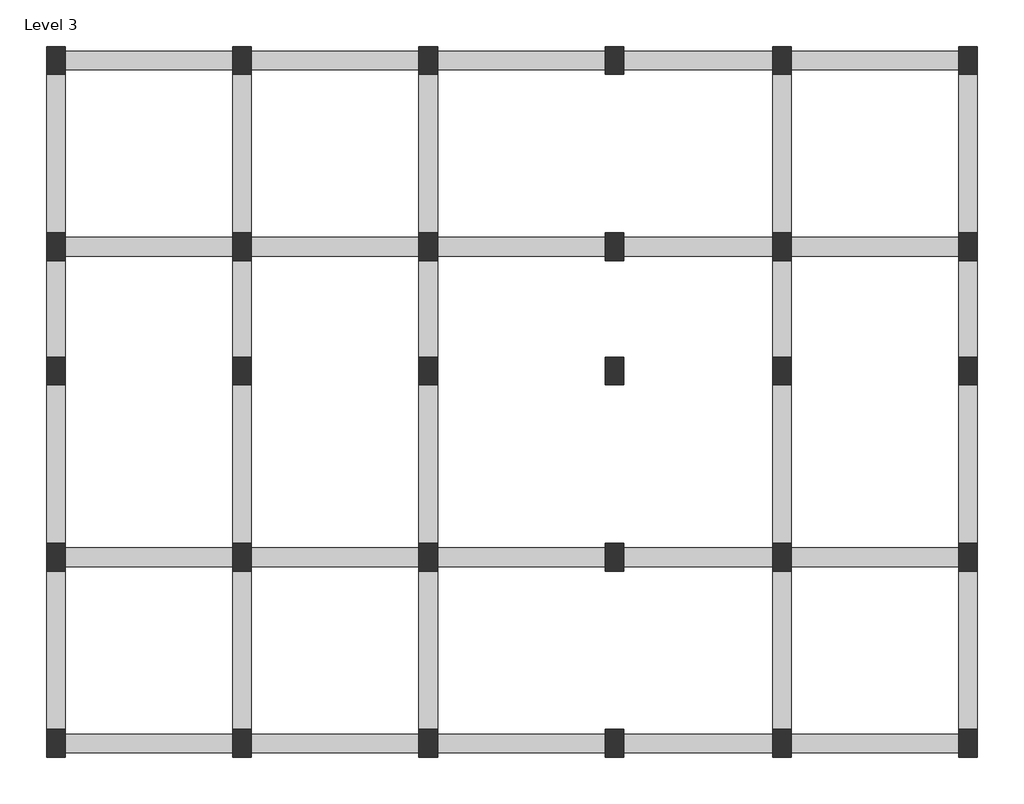
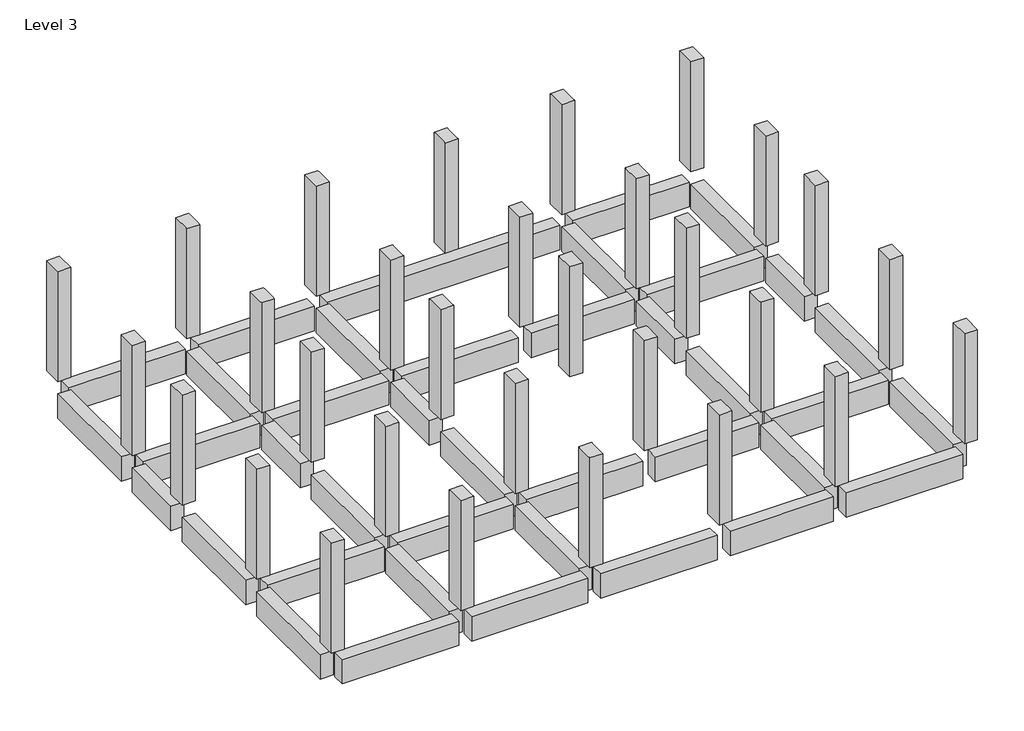
# One storey: 30 columns, 9 beams.
"""IFC4 building model written with IfcOpenShell, lengths in millimetres."""

from ifc_helpers import new_model, si_unit, frame, origin, place, context, project, spatial, polyline, outline, extrude, faceted_brep, element, save

model = new_model("IFC4")

# Units and contexts
model_context = context("Model", 3, world=origin())
ifc_project = project(units=[si_unit("LENGTHUNIT", "METRE", prefix="MILLI")], contexts=[model_context])

# Site, building, storey
site = spatial("IfcSite", under=ifc_project)
building = spatial("IfcBuilding", under=site)
storey = spatial("IfcBuildingStorey", under=building, Name="Level 3", Elevation=6096.0)

# Beams
placement = place(None, origin())
element("IfcBeam", 1, ObjectType="Concrete-Rectangular Beam : 12 x 24", at=placement, inside=storey, context=model_context, shape_type="SweptSolid", body=[
    extrude(outline(polyline([(2607.7603583, 7596.6647757), (2607.7603583, 7291.8647757), (-135.4396417, 7291.8647757), (-135.4396417, 7596.6647757), (2607.7603583, 7596.6647757)])), frame((0.0, 0.0, 5181.6), z_axis=(0.0, 0.0, 1.0), x_axis=(1.0, 0.0, 0.0)), (0.0, 0.0, 1.0), 609.6),
    extrude(outline(polyline([(-12022.6396417, 7291.8647757), (-12022.6396417, 7596.6647757), (-9279.4396417, 7596.6647757), (-9279.4396417, 7291.8647757), (-12022.6396417, 7291.8647757)])), frame((0.0, 0.0, 5181.6), z_axis=(0.0, 0.0, 1.0), x_axis=(1.0, 0.0, 0.0)), (0.0, 0.0, 1.0), 609.6),
    extrude(outline(polyline([(-8974.6396417, 7291.8647757), (-8974.6396417, 7596.6647757), (-6231.4396417, 7596.6647757), (-6231.4396417, 7291.8647757), (-8974.6396417, 7291.8647757)])), frame((0.0, 0.0, 5181.6), z_axis=(0.0, 0.0, 1.0), x_axis=(1.0, 0.0, 0.0)), (0.0, 0.0, 1.0), 609.6),
    extrude(outline(polyline([(-5926.6396417, 7291.8647757), (-5926.6396417, 7596.6647757), (-3183.4396417, 7596.6647757), (-3183.4396417, 7291.8647757), (-5926.6396417, 7291.8647757)])), frame((0.0, 0.0, 5181.6), z_axis=(0.0, 0.0, 1.0), x_axis=(1.0, 0.0, 0.0)), (0.0, 0.0, 1.0), 609.6),
    extrude(outline(polyline([(-2878.6396417, 7291.8647757), (-2878.6396417, 7596.6647757), (-440.2396417, 7596.6647757), (-440.2396417, 7291.8647757), (-2878.6396417, 7291.8647757)])), frame((0.0, 0.0, 5181.6), z_axis=(0.0, 0.0, 1.0), x_axis=(1.0, 0.0, 0.0)), (0.0, 0.0, 1.0), 609.6),
])
element("IfcBeam", 2, ObjectType="Concrete-Rectangular Beam : 12 x 24", at=placement, inside=storey, context=model_context, shape_type="SweptSolid", body=[
    extrude(outline(polyline([(2607.7603583, 10644.6647757), (2607.7603583, 10339.8647757), (-135.4396417, 10339.8647757), (-135.4396417, 10644.6647757), (2607.7603583, 10644.6647757)])), frame((0.0, 0.0, 5181.6), z_axis=(0.0, 0.0, 1.0), x_axis=(1.0, 0.0, 0.0)), (0.0, 0.0, 1.0), 609.6),
    extrude(outline(polyline([(-12022.6396417, 10339.8647757), (-12022.6396417, 10644.6647757), (-9279.4396417, 10644.6647757), (-9279.4396417, 10339.8647757), (-12022.6396417, 10339.8647757)])), frame((0.0, 0.0, 5181.6), z_axis=(0.0, 0.0, 1.0), x_axis=(1.0, 0.0, 0.0)), (0.0, 0.0, 1.0), 609.6),
    extrude(outline(polyline([(-8974.6396417, 10339.8647757), (-8974.6396417, 10644.6647757), (-6231.4396417, 10644.6647757), (-6231.4396417, 10339.8647757), (-8974.6396417, 10339.8647757)])), frame((0.0, 0.0, 5181.6), z_axis=(0.0, 0.0, 1.0), x_axis=(1.0, 0.0, 0.0)), (0.0, 0.0, 1.0), 609.6),
    extrude(outline(polyline([(-5926.6396417, 10339.8647757), (-5926.6396417, 10644.6647757), (-3183.4396417, 10644.6647757), (-3183.4396417, 10339.8647757), (-5926.6396417, 10339.8647757)])), frame((0.0, 0.0, 5181.6), z_axis=(0.0, 0.0, 1.0), x_axis=(1.0, 0.0, 0.0)), (0.0, 0.0, 1.0), 609.6),
    extrude(outline(polyline([(-2878.6396417, 10339.8647757), (-2878.6396417, 10644.6647757), (-440.2396417, 10644.6647757), (-440.2396417, 10339.8647757), (-2878.6396417, 10339.8647757)])), frame((0.0, 0.0, 5181.6), z_axis=(0.0, 0.0, 1.0), x_axis=(1.0, 0.0, 0.0)), (0.0, 0.0, 1.0), 609.6),
])
element("IfcBeam", 3, ObjectType="Concrete-Rectangular Beam : 12 x 24", at=placement, inside=storey, context=model_context, shape_type="SweptSolid", body=[
    extrude(outline(polyline([(2607.7603583, 15727.9119241), (2607.7603583, 15423.1119241), (-135.4396417, 15423.1119241), (-135.4396417, 15727.9119241), (2607.7603583, 15727.9119241)])), frame((0.0, 0.0, 5181.6), z_axis=(0.0, 0.0, 1.0), x_axis=(1.0, 0.0, 0.0)), (0.0, 0.0, 1.0), 609.6),
    extrude(outline(polyline([(-12022.6396417, 15423.1119241), (-12022.6396417, 15727.9119241), (-9279.4396417, 15727.9119241), (-9279.4396417, 15423.1119241), (-12022.6396417, 15423.1119241)])), frame((0.0, 0.0, 5181.6), z_axis=(0.0, 0.0, 1.0), x_axis=(1.0, 0.0, 0.0)), (0.0, 0.0, 1.0), 609.6),
    extrude(outline(polyline([(-8974.6396417, 15423.1119241), (-8974.6396417, 15727.9119241), (-6231.4396417, 15727.9119241), (-6231.4396417, 15423.1119241), (-8974.6396417, 15423.1119241)])), frame((0.0, 0.0, 5181.6), z_axis=(0.0, 0.0, 1.0), x_axis=(1.0, 0.0, 0.0)), (0.0, 0.0, 1.0), 609.6),
    extrude(outline(polyline([(-5926.6396417, 15423.1119241), (-5926.6396417, 15727.9119241), (-3183.4396417, 15727.9119241), (-3183.4396417, 15423.1119241), (-5926.6396417, 15423.1119241)])), frame((0.0, 0.0, 5181.6), z_axis=(0.0, 0.0, 1.0), x_axis=(1.0, 0.0, 0.0)), (0.0, 0.0, 1.0), 609.6),
    extrude(outline(polyline([(-2878.6396417, 15423.1119241), (-2878.6396417, 15727.9119241), (-440.2396417, 15727.9119241), (-440.2396417, 15423.1119241), (-2878.6396417, 15423.1119241)])), frame((0.0, 0.0, 5181.6), z_axis=(0.0, 0.0, 1.0), x_axis=(1.0, 0.0, 0.0)), (0.0, 0.0, 1.0), 609.6),
])
element("IfcBeam", 4, ObjectType="Concrete-Rectangular Beam : 12 x 24", at=placement, inside=storey, context=model_context, shape_type="SweptSolid", body=[
    extrude(outline(polyline([(2607.7603583, 18775.9119241), (2607.7603583, 18471.1119241), (-135.4396417, 18471.1119241), (-135.4396417, 18775.9119241), (2607.7603583, 18775.9119241)])), frame((0.0, 0.0, 5181.6), z_axis=(0.0, 0.0, 1.0), x_axis=(1.0, 0.0, 0.0)), (0.0, 0.0, 1.0), 609.6),
    extrude(outline(polyline([(-12022.6396417, 18471.1119241), (-12022.6396417, 18775.9119241), (-9279.4396417, 18775.9119241), (-9279.4396417, 18471.1119241), (-12022.6396417, 18471.1119241)])), frame((0.0, 0.0, 5181.6), z_axis=(0.0, 0.0, 1.0), x_axis=(1.0, 0.0, 0.0)), (0.0, 0.0, 1.0), 609.6),
    extrude(outline(polyline([(-8974.6396417, 18471.1119241), (-8974.6396417, 18775.9119241), (-6231.4396417, 18775.9119241), (-6231.4396417, 18471.1119241), (-8974.6396417, 18471.1119241)])), frame((0.0, 0.0, 5181.6), z_axis=(0.0, 0.0, 1.0), x_axis=(1.0, 0.0, 0.0)), (0.0, 0.0, 1.0), 609.6),
    extrude(outline(polyline([(-5926.6396417, 18471.1119241), (-5926.6396417, 18775.9119241), (-440.2396417, 18775.9119241), (-440.2396417, 18471.1119241), (-5926.6396417, 18471.1119241)])), frame((0.0, 0.0, 5181.6), z_axis=(0.0, 0.0, 1.0), x_axis=(1.0, 0.0, 0.0)), (0.0, 0.0, 1.0), 609.6),
])
element("IfcBeam", 5, ObjectType="Concrete-Rectangular Beam : 12 x 24", at=placement, inside=storey, context=model_context, shape_type="SweptSolid", body=[
    extrude(outline(polyline([(-12022.6396417, 7672.8647757), (-12327.4396417, 7672.8647757), (-12327.4396417, 10263.6647757), (-12022.6396417, 10263.6647757), (-12022.6396417, 7672.8647757)])), frame((0.0, 0.0, 5181.6), z_axis=(0.0, 0.0, 1.0), x_axis=(1.0, 0.0, 0.0)), (0.0, 0.0, 1.0), 609.6),
    extrude(outline(polyline([(-12327.4396417, 18394.9119241), (-12022.6396417, 18394.9119241), (-12022.6396417, 15804.1119241), (-12327.4396417, 15804.1119241), (-12327.4396417, 18394.9119241)])), frame((0.0, 0.0, 5181.6), z_axis=(0.0, 0.0, 1.0), x_axis=(1.0, 0.0, 0.0)), (0.0, 0.0, 1.0), 609.6),
    extrude(outline(polyline([(-12022.6396417, 10720.8647757), (-12327.4396417, 10720.8647757), (-12327.4396417, 13311.6647757), (-12022.6396417, 13311.6647757), (-12022.6396417, 10720.8647757)])), frame((0.0, 0.0, 5181.6), z_axis=(0.0, 0.0, 1.0), x_axis=(1.0, 0.0, 0.0)), (0.0, 0.0, 1.0), 609.6),
    extrude(outline(polyline([(-12022.6396417, 13768.8647757), (-12327.4396417, 13768.8647757), (-12327.4396417, 15346.9119241), (-12022.6396417, 15346.9119241), (-12022.6396417, 13768.8647757)])), frame((0.0, 0.0, 5181.6), z_axis=(0.0, 0.0, 1.0), x_axis=(1.0, 0.0, 0.0)), (0.0, 0.0, 1.0), 609.6),
])
element("IfcBeam", 6, ObjectType="Concrete-Rectangular Beam : 12 x 24", at=placement, inside=storey, context=model_context, shape_type="SweptSolid", body=[
    extrude(outline(polyline([(-8974.6396417, 7672.8647757), (-9279.4396417, 7672.8647757), (-9279.4396417, 10263.6647757), (-8974.6396417, 10263.6647757), (-8974.6396417, 7672.8647757)])), frame((0.0, 0.0, 5181.6), z_axis=(0.0, 0.0, 1.0), x_axis=(1.0, 0.0, 0.0)), (0.0, 0.0, 1.0), 609.6),
    extrude(outline(polyline([(-9279.4396417, 18394.9119241), (-8974.6396417, 18394.9119241), (-8974.6396417, 15804.1119241), (-9279.4396417, 15804.1119241), (-9279.4396417, 18394.9119241)])), frame((0.0, 0.0, 5181.6), z_axis=(0.0, 0.0, 1.0), x_axis=(1.0, 0.0, 0.0)), (0.0, 0.0, 1.0), 609.6),
    extrude(outline(polyline([(-8974.6396417, 10720.8647757), (-9279.4396417, 10720.8647757), (-9279.4396417, 13311.6647757), (-8974.6396417, 13311.6647757), (-8974.6396417, 10720.8647757)])), frame((0.0, 0.0, 5181.6), z_axis=(0.0, 0.0, 1.0), x_axis=(1.0, 0.0, 0.0)), (0.0, 0.0, 1.0), 609.6),
    extrude(outline(polyline([(-8974.6396417, 13768.8647757), (-9279.4396417, 13768.8647757), (-9279.4396417, 15346.9119241), (-8974.6396417, 15346.9119241), (-8974.6396417, 13768.8647757)])), frame((0.0, 0.0, 5181.6), z_axis=(0.0, 0.0, 1.0), x_axis=(1.0, 0.0, 0.0)), (0.0, 0.0, 1.0), 609.6),
])
element("IfcBeam", 7, ObjectType="Concrete-Rectangular Beam : 12 x 24", at=placement, inside=storey, context=model_context, shape_type="SweptSolid", body=[
    extrude(outline(polyline([(-5926.6396417, 7672.8647757), (-6231.4396417, 7672.8647757), (-6231.4396417, 10263.6647757), (-5926.6396417, 10263.6647757), (-5926.6396417, 7672.8647757)])), frame((0.0, 0.0, 5181.6), z_axis=(0.0, 0.0, 1.0), x_axis=(1.0, 0.0, 0.0)), (0.0, 0.0, 1.0), 609.6),
    extrude(outline(polyline([(-6231.4396417, 18394.9119241), (-5926.6396417, 18394.9119241), (-5926.6396417, 15804.1119241), (-6231.4396417, 15804.1119241), (-6231.4396417, 18394.9119241)])), frame((0.0, 0.0, 5181.6), z_axis=(0.0, 0.0, 1.0), x_axis=(1.0, 0.0, 0.0)), (0.0, 0.0, 1.0), 609.6),
    extrude(outline(polyline([(-5926.6396417, 10720.8647757), (-6231.4396417, 10720.8647757), (-6231.4396417, 13311.6647757), (-5926.6396417, 13311.6647757), (-5926.6396417, 10720.8647757)])), frame((0.0, 0.0, 5181.6), z_axis=(0.0, 0.0, 1.0), x_axis=(1.0, 0.0, 0.0)), (0.0, 0.0, 1.0), 609.6),
    extrude(outline(polyline([(-5926.6396417, 13768.8647757), (-6231.4396417, 13768.8647757), (-6231.4396417, 15346.9119241), (-5926.6396417, 15346.9119241), (-5926.6396417, 13768.8647757)])), frame((0.0, 0.0, 5181.6), z_axis=(0.0, 0.0, 1.0), x_axis=(1.0, 0.0, 0.0)), (0.0, 0.0, 1.0), 609.6),
])
element("IfcBeam", 8, ObjectType="Concrete-Rectangular Beam : 12 x 24", at=placement, inside=storey, context=model_context, shape_type="SweptSolid", body=[
    extrude(outline(polyline([(-135.4396417, 7672.8647757), (-440.2396417, 7672.8647757), (-440.2396417, 10263.6647757), (-135.4396417, 10263.6647757), (-135.4396417, 7672.8647757)])), frame((0.0, 0.0, 5181.6), z_axis=(0.0, 0.0, 1.0), x_axis=(1.0, 0.0, 0.0)), (0.0, 0.0, 1.0), 609.6),
    extrude(outline(polyline([(-440.2396417, 18394.9119241), (-135.4396417, 18394.9119241), (-135.4396417, 15804.1119241), (-440.2396417, 15804.1119241), (-440.2396417, 18394.9119241)])), frame((0.0, 0.0, 5181.6), z_axis=(0.0, 0.0, 1.0), x_axis=(1.0, 0.0, 0.0)), (0.0, 0.0, 1.0), 609.6),
    extrude(outline(polyline([(-135.4396417, 10720.8647757), (-440.2396417, 10720.8647757), (-440.2396417, 13311.6647757), (-135.4396417, 13311.6647757), (-135.4396417, 10720.8647757)])), frame((0.0, 0.0, 5181.6), z_axis=(0.0, 0.0, 1.0), x_axis=(1.0, 0.0, 0.0)), (0.0, 0.0, 1.0), 609.6),
    extrude(outline(polyline([(-135.4396417, 13768.8647757), (-440.2396417, 13768.8647757), (-440.2396417, 15346.9119241), (-135.4396417, 15346.9119241), (-135.4396417, 13768.8647757)])), frame((0.0, 0.0, 5181.6), z_axis=(0.0, 0.0, 1.0), x_axis=(1.0, 0.0, 0.0)), (0.0, 0.0, 1.0), 609.6),
])
element("IfcBeam", 9, ObjectType="Concrete-Rectangular Beam : 12 x 24", at=placement, inside=storey, context=model_context, shape_type="SweptSolid", body=[
    extrude(outline(polyline([(2912.5603583, 7672.8647757), (2607.7603583, 7672.8647757), (2607.7603583, 10263.6647757), (2912.5603583, 10263.6647757), (2912.5603583, 7672.8647757)])), frame((0.0, 0.0, 5181.6), z_axis=(0.0, 0.0, 1.0), x_axis=(1.0, 0.0, 0.0)), (0.0, 0.0, 1.0), 609.6),
    extrude(outline(polyline([(2607.7603583, 18394.9119241), (2912.5603583, 18394.9119241), (2912.5603583, 15804.1119241), (2607.7603583, 15804.1119241), (2607.7603583, 18394.9119241)])), frame((0.0, 0.0, 5181.6), z_axis=(0.0, 0.0, 1.0), x_axis=(1.0, 0.0, 0.0)), (0.0, 0.0, 1.0), 609.6),
    extrude(outline(polyline([(2912.5603583, 10720.8647757), (2607.7603583, 10720.8647757), (2607.7603583, 13311.6647757), (2912.5603583, 13311.6647757), (2912.5603583, 10720.8647757)])), frame((0.0, 0.0, 5181.6), z_axis=(0.0, 0.0, 1.0), x_axis=(1.0, 0.0, 0.0)), (0.0, 0.0, 1.0), 609.6),
    extrude(outline(polyline([(2912.5603583, 13768.8647757), (2607.7603583, 13768.8647757), (2607.7603583, 15346.9119241), (2912.5603583, 15346.9119241), (2912.5603583, 13768.8647757)])), frame((0.0, 0.0, 5181.6), z_axis=(0.0, 0.0, 1.0), x_axis=(1.0, 0.0, 0.0)), (0.0, 0.0, 1.0), 609.6),
])

# Columns
element("IfcColumn", 10, ObjectType="Concrete-Rectangular-Column : c1", at=placement, inside=storey, context=model_context, shape_type="SweptSolid", body=[
    extrude(outline(polyline([(-12327.4396417, 7215.6647757), (-12327.4396417, 7672.8647757), (-12022.6396417, 7672.8647757), (-12022.6396417, 7215.6647757), (-12327.4396417, 7215.6647757)])), frame((0.0, 0.0, 6096.0), z_axis=(0.0, 0.0, 1.0), x_axis=(1.0, 0.0, 0.0)), (0.0, 0.0, 1.0), 2743.2),
])
element("IfcColumn", 11, ObjectType="Concrete-Rectangular-Column : c1", at=placement, inside=storey, context=model_context, shape_type="Brep", body=[
    faceted_brep([(-9279.4396417, 7215.6647757, 6096.0), (-9279.4396417, 7672.8647757, 6096.0), (-8974.6396417, 7672.8647757, 6096.0), (-8974.6396417, 7215.6647757, 6096.0), (-9279.4396417, 7215.6647757, 8839.2), (-9279.4396417, 7291.8647757, 8839.2), (-9279.4396417, 7596.6647757, 8839.2), (-9279.4396417, 7672.8647757, 8839.2), (-8974.6396417, 7672.8647757, 8839.2), (-8974.6396417, 7596.6647757, 8839.2), (-8974.6396417, 7291.8647757, 8839.2), (-8974.6396417, 7215.6647757, 8839.2)], [[[0, 1, 2, 3]], [[4, 5, 6, 7, 1, 0]], [[7, 8, 2, 1]], [[8, 9, 10, 11, 3, 2]], [[11, 4, 0, 3]], [[4, 11, 10, 9, 8, 7, 6, 5]]]),
])
element("IfcColumn", 12, ObjectType="Concrete-Rectangular-Column : c1", at=placement, inside=storey, context=model_context, shape_type="Brep", body=[
    faceted_brep([(-6231.4396417, 7215.6647757, 6096.0), (-6231.4396417, 7672.8647757, 6096.0), (-5926.6396417, 7672.8647757, 6096.0), (-5926.6396417, 7215.6647757, 6096.0), (-6231.4396417, 7215.6647757, 8839.2), (-6231.4396417, 7291.8647757, 8839.2), (-6231.4396417, 7596.6647757, 8839.2), (-6231.4396417, 7672.8647757, 8839.2), (-5926.6396417, 7672.8647757, 8839.2), (-5926.6396417, 7596.6647757, 8839.2), (-5926.6396417, 7291.8647757, 8839.2), (-5926.6396417, 7215.6647757, 8839.2)], [[[0, 1, 2, 3]], [[4, 5, 6, 7, 1, 0]], [[7, 8, 2, 1]], [[8, 9, 10, 11, 3, 2]], [[11, 4, 0, 3]], [[4, 11, 10, 9, 8, 7, 6, 5]]]),
])
element("IfcColumn", 13, ObjectType="Concrete-Rectangular-Column : c1", at=placement, inside=storey, context=model_context, shape_type="Brep", body=[
    faceted_brep([(-3183.4396417, 7215.6647757, 6096.0), (-3183.4396417, 7672.8647757, 6096.0), (-2878.6396417, 7672.8647757, 6096.0), (-2878.6396417, 7215.6647757, 6096.0), (-3183.4396417, 7215.6647757, 8839.2), (-3183.4396417, 7291.8647757, 8839.2), (-3183.4396417, 7596.6647757, 8839.2), (-3183.4396417, 7672.8647757, 8839.2), (-2878.6396417, 7672.8647757, 8839.2), (-2878.6396417, 7596.6647757, 8839.2), (-2878.6396417, 7291.8647757, 8839.2), (-2878.6396417, 7215.6647757, 8839.2)], [[[0, 1, 2, 3]], [[4, 5, 6, 7, 1, 0]], [[7, 8, 2, 1]], [[8, 9, 10, 11, 3, 2]], [[11, 4, 0, 3]], [[4, 11, 10, 9, 8, 7, 6, 5]]]),
])
element("IfcColumn", 14, ObjectType="Concrete-Rectangular-Column : c1", at=placement, inside=storey, context=model_context, shape_type="Brep", body=[
    faceted_brep([(-440.2396417, 7215.6647757, 6096.0), (-440.2396417, 7672.8647757, 6096.0), (-135.4396417, 7672.8647757, 6096.0), (-135.4396417, 7215.6647757, 6096.0), (-440.2396417, 7215.6647757, 8839.2), (-440.2396417, 7291.8647757, 8839.2), (-440.2396417, 7596.6647757, 8839.2), (-440.2396417, 7672.8647757, 8839.2), (-135.4396417, 7672.8647757, 8839.2), (-135.4396417, 7596.6647757, 8839.2), (-135.4396417, 7291.8647757, 8839.2), (-135.4396417, 7215.6647757, 8839.2)], [[[0, 1, 2, 3]], [[4, 5, 6, 7, 1, 0]], [[7, 8, 2, 1]], [[8, 9, 10, 11, 3, 2]], [[11, 4, 0, 3]], [[4, 11, 10, 9, 8, 7, 6, 5]]]),
])
element("IfcColumn", 15, ObjectType="Concrete-Rectangular-Column : c1", at=placement, inside=storey, context=model_context, shape_type="SweptSolid", body=[
    extrude(outline(polyline([(2607.7603583, 7215.6647757), (2607.7603583, 7672.8647757), (2912.5603583, 7672.8647757), (2912.5603583, 7215.6647757), (2607.7603583, 7215.6647757)])), frame((0.0, 0.0, 6096.0), z_axis=(0.0, 0.0, 1.0), x_axis=(1.0, 0.0, 0.0)), (0.0, 0.0, 1.0), 2743.2),
])
element("IfcColumn", 16, ObjectType="Concrete-Rectangular-Column : c1", at=placement, inside=storey, context=model_context, shape_type="Brep", body=[
    faceted_brep([(-12327.4396417, 10263.6647757, 6096.0), (-12327.4396417, 10720.8647757, 6096.0), (-12022.6396417, 10720.8647757, 6096.0), (-12022.6396417, 10263.6647757, 6096.0), (-12327.4396417, 10263.6647757, 8839.2), (-12327.4396417, 10720.8647757, 8839.2), (-12327.4396417, 10720.8647757, 8229.6), (-12327.4396417, 10263.6647757, 8229.6), (-12022.6396417, 10720.8647757, 8839.2), (-12022.6396417, 10720.8647757, 8229.6), (-12022.6396417, 10263.6647757, 8839.2), (-12022.6396417, 10263.6647757, 8229.6)], [[[0, 1, 2, 3]], [[4, 5, 6, 1, 0, 7]], [[5, 8, 9, 2, 1, 6]], [[8, 10, 11, 3, 2, 9]], [[10, 4, 7, 0, 3, 11]], [[4, 10, 8, 5]]]),
])
element("IfcColumn", 17, ObjectType="Concrete-Rectangular-Column : c1", at=placement, inside=storey, context=model_context, shape_type="Brep", body=[
    faceted_brep([(-9279.4396417, 10263.6647757, 6096.0), (-9279.4396417, 10720.8647757, 6096.0), (-8974.6396417, 10720.8647757, 6096.0), (-8974.6396417, 10263.6647757, 6096.0), (-9279.4396417, 10263.6647757, 8839.2), (-9279.4396417, 10339.8647757, 8839.2), (-9279.4396417, 10644.6647757, 8839.2), (-9279.4396417, 10720.8647757, 8839.2), (-9279.4396417, 10720.8647757, 8229.6), (-9279.4396417, 10263.6647757, 8229.6), (-8974.6396417, 10720.8647757, 8839.2), (-8974.6396417, 10720.8647757, 8229.6), (-8974.6396417, 10644.6647757, 8839.2), (-8974.6396417, 10339.8647757, 8839.2), (-8974.6396417, 10263.6647757, 8839.2), (-8974.6396417, 10263.6647757, 8229.6)], [[[0, 1, 2, 3]], [[4, 5, 6, 7, 8, 1, 0, 9]], [[7, 10, 11, 2, 1, 8]], [[10, 12, 13, 14, 15, 3, 2, 11]], [[14, 4, 9, 0, 3, 15]], [[4, 14, 13, 12, 10, 7, 6, 5]]]),
])
element("IfcColumn", 18, ObjectType="Concrete-Rectangular-Column : c1", at=placement, inside=storey, context=model_context, shape_type="Brep", body=[
    faceted_brep([(-6231.4396417, 10263.6647757, 6096.0), (-6231.4396417, 10720.8647757, 6096.0), (-5926.6396417, 10720.8647757, 6096.0), (-5926.6396417, 10263.6647757, 6096.0), (-6231.4396417, 10263.6647757, 8839.2), (-6231.4396417, 10339.8647757, 8839.2), (-6231.4396417, 10644.6647757, 8839.2), (-6231.4396417, 10720.8647757, 8839.2), (-6231.4396417, 10720.8647757, 8229.6), (-6231.4396417, 10263.6647757, 8229.6), (-5926.6396417, 10720.8647757, 8839.2), (-5926.6396417, 10720.8647757, 8229.6), (-5926.6396417, 10644.6647757, 8839.2), (-5926.6396417, 10339.8647757, 8839.2), (-5926.6396417, 10263.6647757, 8839.2), (-5926.6396417, 10263.6647757, 8229.6)], [[[0, 1, 2, 3]], [[4, 5, 6, 7, 8, 1, 0, 9]], [[7, 10, 11, 2, 1, 8]], [[10, 12, 13, 14, 15, 3, 2, 11]], [[14, 4, 9, 0, 3, 15]], [[4, 14, 13, 12, 10, 7, 6, 5]]]),
])
element("IfcColumn", 19, ObjectType="Concrete-Rectangular-Column : c1", at=placement, inside=storey, context=model_context, shape_type="Brep", body=[
    faceted_brep([(-3183.4396417, 10263.6647757, 6096.0), (-3183.4396417, 10720.8647757, 6096.0), (-2878.6396417, 10720.8647757, 6096.0), (-2878.6396417, 10263.6647757, 6096.0), (-3183.4396417, 10263.6647757, 8839.2), (-3183.4396417, 10339.8647757, 8839.2), (-3183.4396417, 10644.6647757, 8839.2), (-3183.4396417, 10720.8647757, 8839.2), (-3183.4396417, 10720.8647757, 8229.6), (-3183.4396417, 10263.6647757, 8229.6), (-2878.6396417, 10720.8647757, 8839.2), (-2878.6396417, 10720.8647757, 8229.6), (-2878.6396417, 10644.6647757, 8839.2), (-2878.6396417, 10339.8647757, 8839.2), (-2878.6396417, 10263.6647757, 8839.2), (-2878.6396417, 10263.6647757, 8229.6)], [[[0, 1, 2, 3]], [[4, 5, 6, 7, 8, 1, 0, 9]], [[7, 10, 11, 2, 1, 8]], [[10, 12, 13, 14, 15, 3, 2, 11]], [[14, 4, 9, 0, 3, 15]], [[4, 14, 13, 12, 10, 7, 6, 5]]]),
])
element("IfcColumn", 20, ObjectType="Concrete-Rectangular-Column : c1", at=placement, inside=storey, context=model_context, shape_type="Brep", body=[
    faceted_brep([(-440.2396417, 10263.6647757, 6096.0), (-440.2396417, 10720.8647757, 6096.0), (-135.4396417, 10720.8647757, 6096.0), (-135.4396417, 10263.6647757, 6096.0), (-440.2396417, 10263.6647757, 8839.2), (-440.2396417, 10339.8647757, 8839.2), (-440.2396417, 10644.6647757, 8839.2), (-440.2396417, 10720.8647757, 8839.2), (-440.2396417, 10720.8647757, 8229.6), (-440.2396417, 10263.6647757, 8229.6), (-135.4396417, 10720.8647757, 8839.2), (-135.4396417, 10720.8647757, 8229.6), (-135.4396417, 10644.6647757, 8839.2), (-135.4396417, 10339.8647757, 8839.2), (-135.4396417, 10263.6647757, 8839.2), (-135.4396417, 10263.6647757, 8229.6)], [[[0, 1, 2, 3]], [[4, 5, 6, 7, 8, 1, 0, 9]], [[7, 10, 11, 2, 1, 8]], [[10, 12, 13, 14, 15, 3, 2, 11]], [[14, 4, 9, 0, 3, 15]], [[4, 14, 13, 12, 10, 7, 6, 5]]]),
])
element("IfcColumn", 21, ObjectType="Concrete-Rectangular-Column : c1", at=placement, inside=storey, context=model_context, shape_type="Brep", body=[
    faceted_brep([(2607.7603583, 10263.6647757, 6096.0), (2607.7603583, 10720.8647757, 6096.0), (2912.5603583, 10720.8647757, 6096.0), (2912.5603583, 10263.6647757, 6096.0), (2607.7603583, 10263.6647757, 8839.2), (2607.7603583, 10720.8647757, 8839.2), (2607.7603583, 10720.8647757, 8229.6), (2607.7603583, 10263.6647757, 8229.6), (2912.5603583, 10720.8647757, 8839.2), (2912.5603583, 10720.8647757, 8229.6), (2912.5603583, 10263.6647757, 8839.2), (2912.5603583, 10263.6647757, 8229.6)], [[[0, 1, 2, 3]], [[4, 5, 6, 1, 0, 7]], [[5, 8, 9, 2, 1, 6]], [[8, 10, 11, 3, 2, 9]], [[10, 4, 7, 0, 3, 11]], [[4, 10, 8, 5]]]),
])
element("IfcColumn", 22, ObjectType="Concrete-Rectangular-Column : c1", at=placement, inside=storey, context=model_context, shape_type="Brep", body=[
    faceted_brep([(-12327.4396417, 13311.6647757, 6096.0), (-12327.4396417, 13768.8647757, 6096.0), (-12022.6396417, 13768.8647757, 6096.0), (-12022.6396417, 13311.6647757, 6096.0), (-12327.4396417, 13311.6647757, 8839.2), (-12327.4396417, 13768.8647757, 8839.2), (-12327.4396417, 13768.8647757, 8229.6), (-12327.4396417, 13311.6647757, 8229.6), (-12022.6396417, 13768.8647757, 8839.2), (-12022.6396417, 13768.8647757, 8229.6), (-12022.6396417, 13311.6647757, 8839.2), (-12022.6396417, 13311.6647757, 8229.6)], [[[0, 1, 2, 3]], [[4, 5, 6, 1, 0, 7]], [[5, 8, 9, 2, 1, 6]], [[8, 10, 11, 3, 2, 9]], [[10, 4, 7, 0, 3, 11]], [[4, 10, 8, 5]]]),
])
element("IfcColumn", 23, ObjectType="Concrete-Rectangular-Column : c1", at=placement, inside=storey, context=model_context, shape_type="Brep", body=[
    faceted_brep([(-9279.4396417, 13311.6647757, 6096.0), (-9279.4396417, 13768.8647757, 6096.0), (-8974.6396417, 13768.8647757, 6096.0), (-8974.6396417, 13311.6647757, 6096.0), (-9279.4396417, 13311.6647757, 8839.2), (-9279.4396417, 13387.8647757, 8839.2), (-9279.4396417, 13692.6647757, 8839.2), (-9279.4396417, 13768.8647757, 8839.2), (-9279.4396417, 13768.8647757, 8229.6), (-9279.4396417, 13311.6647757, 8229.6), (-8974.6396417, 13768.8647757, 8839.2), (-8974.6396417, 13768.8647757, 8229.6), (-8974.6396417, 13692.6647757, 8839.2), (-8974.6396417, 13387.8647757, 8839.2), (-8974.6396417, 13311.6647757, 8839.2), (-8974.6396417, 13311.6647757, 8229.6)], [[[0, 1, 2, 3]], [[4, 5, 6, 7, 8, 1, 0, 9]], [[7, 10, 11, 2, 1, 8]], [[10, 12, 13, 14, 15, 3, 2, 11]], [[14, 4, 9, 0, 3, 15]], [[4, 14, 13, 12, 10, 7, 6, 5]]]),
])
element("IfcColumn", 24, ObjectType="Concrete-Rectangular-Column : c1", at=placement, inside=storey, context=model_context, shape_type="Brep", body=[
    faceted_brep([(-6231.4396417, 13311.6647757, 6096.0), (-6231.4396417, 13768.8647757, 6096.0), (-5926.6396417, 13768.8647757, 6096.0), (-5926.6396417, 13311.6647757, 6096.0), (-6231.4396417, 13311.6647757, 8839.2), (-6231.4396417, 13387.8647757, 8839.2), (-6231.4396417, 13692.6647757, 8839.2), (-6231.4396417, 13768.8647757, 8839.2), (-6231.4396417, 13768.8647757, 8229.6), (-6231.4396417, 13311.6647757, 8229.6), (-5926.6396417, 13768.8647757, 8839.2), (-5926.6396417, 13768.8647757, 8229.6), (-5926.6396417, 13692.6647757, 8839.2), (-5926.6396417, 13387.8647757, 8839.2), (-5926.6396417, 13311.6647757, 8839.2), (-5926.6396417, 13311.6647757, 8229.6)], [[[0, 1, 2, 3]], [[4, 5, 6, 7, 8, 1, 0, 9]], [[7, 10, 11, 2, 1, 8]], [[10, 12, 13, 14, 15, 3, 2, 11]], [[14, 4, 9, 0, 3, 15]], [[4, 14, 13, 12, 10, 7, 6, 5]]]),
])
element("IfcColumn", 25, ObjectType="Concrete-Rectangular-Column : c1", at=placement, inside=storey, context=model_context, shape_type="Brep", body=[
    faceted_brep([(-3183.4396417, 13311.6647757, 6096.0), (-3183.4396417, 13768.8647757, 6096.0), (-2878.6396417, 13768.8647757, 6096.0), (-2878.6396417, 13311.6647757, 6096.0), (-3183.4396417, 13311.6647757, 8839.2), (-3183.4396417, 13387.8647757, 8839.2), (-3183.4396417, 13692.6647757, 8839.2), (-3183.4396417, 13768.8647757, 8839.2), (-3183.4396417, 13768.8647757, 8229.6), (-3183.4396417, 13311.6647757, 8229.6), (-2878.6396417, 13768.8647757, 8839.2), (-2878.6396417, 13768.8647757, 8229.6), (-2878.6396417, 13692.6647757, 8839.2), (-2878.6396417, 13387.8647757, 8839.2), (-2878.6396417, 13311.6647757, 8839.2), (-2878.6396417, 13311.6647757, 8229.6)], [[[0, 1, 2, 3]], [[4, 5, 6, 7, 8, 1, 0, 9]], [[7, 10, 11, 2, 1, 8]], [[10, 12, 13, 14, 15, 3, 2, 11]], [[14, 4, 9, 0, 3, 15]], [[4, 14, 13, 12, 10, 7, 6, 5]]]),
])
element("IfcColumn", 26, ObjectType="Concrete-Rectangular-Column : c1", at=placement, inside=storey, context=model_context, shape_type="Brep", body=[
    faceted_brep([(-440.2396417, 13311.6647757, 6096.0), (-440.2396417, 13768.8647757, 6096.0), (-135.4396417, 13768.8647757, 6096.0), (-135.4396417, 13311.6647757, 6096.0), (-440.2396417, 13311.6647757, 8839.2), (-440.2396417, 13387.8647757, 8839.2), (-440.2396417, 13692.6647757, 8839.2), (-440.2396417, 13768.8647757, 8839.2), (-440.2396417, 13768.8647757, 8229.6), (-440.2396417, 13311.6647757, 8229.6), (-135.4396417, 13768.8647757, 8839.2), (-135.4396417, 13768.8647757, 8229.6), (-135.4396417, 13692.6647757, 8839.2), (-135.4396417, 13387.8647757, 8839.2), (-135.4396417, 13311.6647757, 8839.2), (-135.4396417, 13311.6647757, 8229.6)], [[[0, 1, 2, 3]], [[4, 5, 6, 7, 8, 1, 0, 9]], [[7, 10, 11, 2, 1, 8]], [[10, 12, 13, 14, 15, 3, 2, 11]], [[14, 4, 9, 0, 3, 15]], [[4, 14, 13, 12, 10, 7, 6, 5]]]),
])
element("IfcColumn", 27, ObjectType="Concrete-Rectangular-Column : c1", at=placement, inside=storey, context=model_context, shape_type="Brep", body=[
    faceted_brep([(2607.7603583, 13311.6647757, 6096.0), (2607.7603583, 13768.8647757, 6096.0), (2912.5603583, 13768.8647757, 6096.0), (2912.5603583, 13311.6647757, 6096.0), (2607.7603583, 13311.6647757, 8839.2), (2607.7603583, 13768.8647757, 8839.2), (2607.7603583, 13768.8647757, 8229.6), (2607.7603583, 13311.6647757, 8229.6), (2912.5603583, 13768.8647757, 8839.2), (2912.5603583, 13768.8647757, 8229.6), (2912.5603583, 13311.6647757, 8839.2), (2912.5603583, 13311.6647757, 8229.6)], [[[0, 1, 2, 3]], [[4, 5, 6, 1, 0, 7]], [[5, 8, 9, 2, 1, 6]], [[8, 10, 11, 3, 2, 9]], [[10, 4, 7, 0, 3, 11]], [[4, 10, 8, 5]]]),
])
element("IfcColumn", 28, ObjectType="Concrete-Rectangular-Column : c1", at=placement, inside=storey, context=model_context, shape_type="Brep", body=[
    faceted_brep([(-12327.4396417, 15346.9119241, 6096.0), (-12327.4396417, 15804.1119241, 6096.0), (-12022.6396417, 15804.1119241, 6096.0), (-12022.6396417, 15346.9119241, 6096.0), (-12327.4396417, 15346.9119241, 8839.2), (-12327.4396417, 15804.1119241, 8839.2), (-12327.4396417, 15804.1119241, 8229.6), (-12327.4396417, 15346.9119241, 8229.6), (-12022.6396417, 15804.1119241, 8839.2), (-12022.6396417, 15804.1119241, 8229.6), (-12022.6396417, 15346.9119241, 8839.2), (-12022.6396417, 15346.9119241, 8229.6)], [[[0, 1, 2, 3]], [[4, 5, 6, 1, 0, 7]], [[5, 8, 9, 2, 1, 6]], [[8, 10, 11, 3, 2, 9]], [[10, 4, 7, 0, 3, 11]], [[4, 10, 8, 5]]]),
])
element("IfcColumn", 29, ObjectType="Concrete-Rectangular-Column : c1", at=placement, inside=storey, context=model_context, shape_type="Brep", body=[
    faceted_brep([(-9279.4396417, 15346.9119241, 6096.0), (-9279.4396417, 15804.1119241, 6096.0), (-8974.6396417, 15804.1119241, 6096.0), (-8974.6396417, 15346.9119241, 6096.0), (-9279.4396417, 15346.9119241, 8839.2), (-9279.4396417, 15423.1119241, 8839.2), (-9279.4396417, 15727.9119241, 8839.2), (-9279.4396417, 15804.1119241, 8839.2), (-9279.4396417, 15804.1119241, 8229.6), (-9279.4396417, 15346.9119241, 8229.6), (-8974.6396417, 15804.1119241, 8839.2), (-8974.6396417, 15804.1119241, 8229.6), (-8974.6396417, 15727.9119241, 8839.2), (-8974.6396417, 15423.1119241, 8839.2), (-8974.6396417, 15346.9119241, 8839.2), (-8974.6396417, 15346.9119241, 8229.6)], [[[0, 1, 2, 3]], [[4, 5, 6, 7, 8, 1, 0, 9]], [[7, 10, 11, 2, 1, 8]], [[10, 12, 13, 14, 15, 3, 2, 11]], [[14, 4, 9, 0, 3, 15]], [[4, 14, 13, 12, 10, 7, 6, 5]]]),
])
element("IfcColumn", 30, ObjectType="Concrete-Rectangular-Column : c1", at=placement, inside=storey, context=model_context, shape_type="Brep", body=[
    faceted_brep([(-6231.4396417, 15346.9119241, 6096.0), (-6231.4396417, 15804.1119241, 6096.0), (-5926.6396417, 15804.1119241, 6096.0), (-5926.6396417, 15346.9119241, 6096.0), (-6231.4396417, 15346.9119241, 8839.2), (-6231.4396417, 15423.1119241, 8839.2), (-6231.4396417, 15727.9119241, 8839.2), (-6231.4396417, 15804.1119241, 8839.2), (-6231.4396417, 15804.1119241, 8229.6), (-6231.4396417, 15346.9119241, 8229.6), (-5926.6396417, 15804.1119241, 8839.2), (-5926.6396417, 15804.1119241, 8229.6), (-5926.6396417, 15727.9119241, 8839.2), (-5926.6396417, 15423.1119241, 8839.2), (-5926.6396417, 15346.9119241, 8839.2), (-5926.6396417, 15346.9119241, 8229.6)], [[[0, 1, 2, 3]], [[4, 5, 6, 7, 8, 1, 0, 9]], [[7, 10, 11, 2, 1, 8]], [[10, 12, 13, 14, 15, 3, 2, 11]], [[14, 4, 9, 0, 3, 15]], [[4, 14, 13, 12, 10, 7, 6, 5]]]),
])
element("IfcColumn", 31, ObjectType="Concrete-Rectangular-Column : c1", at=placement, inside=storey, context=model_context, shape_type="Brep", body=[
    faceted_brep([(-3183.4396417, 15346.9119241, 6096.0), (-3183.4396417, 15804.1119241, 6096.0), (-2878.6396417, 15804.1119241, 6096.0), (-2878.6396417, 15346.9119241, 6096.0), (-3183.4396417, 15346.9119241, 8839.2), (-3183.4396417, 15423.1119241, 8839.2), (-3183.4396417, 15727.9119241, 8839.2), (-3183.4396417, 15804.1119241, 8839.2), (-3183.4396417, 15804.1119241, 8229.6), (-3183.4396417, 15346.9119241, 8229.6), (-2878.6396417, 15804.1119241, 8839.2), (-2878.6396417, 15804.1119241, 8229.6), (-2878.6396417, 15727.9119241, 8839.2), (-2878.6396417, 15423.1119241, 8839.2), (-2878.6396417, 15346.9119241, 8839.2), (-2878.6396417, 15346.9119241, 8229.6)], [[[0, 1, 2, 3]], [[4, 5, 6, 7, 8, 1, 0, 9]], [[7, 10, 11, 2, 1, 8]], [[10, 12, 13, 14, 15, 3, 2, 11]], [[14, 4, 9, 0, 3, 15]], [[4, 14, 13, 12, 10, 7, 6, 5]]]),
])
element("IfcColumn", 32, ObjectType="Concrete-Rectangular-Column : c1", at=placement, inside=storey, context=model_context, shape_type="Brep", body=[
    faceted_brep([(-440.2396417, 15346.9119241, 6096.0), (-440.2396417, 15804.1119241, 6096.0), (-135.4396417, 15804.1119241, 6096.0), (-135.4396417, 15346.9119241, 6096.0), (-440.2396417, 15346.9119241, 8839.2), (-440.2396417, 15423.1119241, 8839.2), (-440.2396417, 15727.9119241, 8839.2), (-440.2396417, 15804.1119241, 8839.2), (-440.2396417, 15804.1119241, 8229.6), (-440.2396417, 15346.9119241, 8229.6), (-135.4396417, 15804.1119241, 8839.2), (-135.4396417, 15804.1119241, 8229.6), (-135.4396417, 15727.9119241, 8839.2), (-135.4396417, 15423.1119241, 8839.2), (-135.4396417, 15346.9119241, 8839.2), (-135.4396417, 15346.9119241, 8229.6)], [[[0, 1, 2, 3]], [[4, 5, 6, 7, 8, 1, 0, 9]], [[7, 10, 11, 2, 1, 8]], [[10, 12, 13, 14, 15, 3, 2, 11]], [[14, 4, 9, 0, 3, 15]], [[4, 14, 13, 12, 10, 7, 6, 5]]]),
])
element("IfcColumn", 33, ObjectType="Concrete-Rectangular-Column : c1", at=placement, inside=storey, context=model_context, shape_type="Brep", body=[
    faceted_brep([(2607.7603583, 15346.9119241, 6096.0), (2607.7603583, 15804.1119241, 6096.0), (2912.5603583, 15804.1119241, 6096.0), (2912.5603583, 15346.9119241, 6096.0), (2607.7603583, 15346.9119241, 8839.2), (2607.7603583, 15804.1119241, 8839.2), (2607.7603583, 15804.1119241, 8229.6), (2607.7603583, 15346.9119241, 8229.6), (2912.5603583, 15804.1119241, 8839.2), (2912.5603583, 15804.1119241, 8229.6), (2912.5603583, 15346.9119241, 8839.2), (2912.5603583, 15346.9119241, 8229.6)], [[[0, 1, 2, 3]], [[4, 5, 6, 1, 0, 7]], [[5, 8, 9, 2, 1, 6]], [[8, 10, 11, 3, 2, 9]], [[10, 4, 7, 0, 3, 11]], [[4, 10, 8, 5]]]),
])
element("IfcColumn", 34, ObjectType="Concrete-Rectangular-Column : c1", at=placement, inside=storey, context=model_context, shape_type="SweptSolid", body=[
    extrude(outline(polyline([(-12327.4396417, 18394.9119241), (-12327.4396417, 18852.1119241), (-12022.6396417, 18852.1119241), (-12022.6396417, 18394.9119241), (-12327.4396417, 18394.9119241)])), frame((0.0, 0.0, 6096.0), z_axis=(0.0, 0.0, 1.0), x_axis=(1.0, 0.0, 0.0)), (0.0, 0.0, 1.0), 2743.2),
])
element("IfcColumn", 35, ObjectType="Concrete-Rectangular-Column : c1", at=placement, inside=storey, context=model_context, shape_type="Brep", body=[
    faceted_brep([(-9279.4396417, 18394.9119241, 6096.0), (-9279.4396417, 18852.1119241, 6096.0), (-8974.6396417, 18852.1119241, 6096.0), (-8974.6396417, 18394.9119241, 6096.0), (-9279.4396417, 18394.9119241, 8839.2), (-9279.4396417, 18471.1119241, 8839.2), (-9279.4396417, 18775.9119241, 8839.2), (-9279.4396417, 18852.1119241, 8839.2), (-8974.6396417, 18852.1119241, 8839.2), (-8974.6396417, 18775.9119241, 8839.2), (-8974.6396417, 18471.1119241, 8839.2), (-8974.6396417, 18394.9119241, 8839.2)], [[[0, 1, 2, 3]], [[4, 5, 6, 7, 1, 0]], [[7, 8, 2, 1]], [[8, 9, 10, 11, 3, 2]], [[11, 4, 0, 3]], [[4, 11, 10, 9, 8, 7, 6, 5]]]),
])
element("IfcColumn", 36, ObjectType="Concrete-Rectangular-Column : c1", at=placement, inside=storey, context=model_context, shape_type="Brep", body=[
    faceted_brep([(-6231.4396417, 18394.9119241, 6096.0), (-6231.4396417, 18852.1119241, 6096.0), (-5926.6396417, 18852.1119241, 6096.0), (-5926.6396417, 18394.9119241, 6096.0), (-6231.4396417, 18394.9119241, 8839.2), (-6231.4396417, 18471.1119241, 8839.2), (-6231.4396417, 18775.9119241, 8839.2), (-6231.4396417, 18852.1119241, 8839.2), (-5926.6396417, 18852.1119241, 8839.2), (-5926.6396417, 18775.9119241, 8839.2), (-5926.6396417, 18471.1119241, 8839.2), (-5926.6396417, 18394.9119241, 8839.2)], [[[0, 1, 2, 3]], [[4, 5, 6, 7, 1, 0]], [[7, 8, 2, 1]], [[8, 9, 10, 11, 3, 2]], [[11, 4, 0, 3]], [[4, 11, 10, 9, 8, 7, 6, 5]]]),
])
element("IfcColumn", 37, ObjectType="Concrete-Rectangular-Column : c1", at=placement, inside=storey, context=model_context, shape_type="Brep", body=[
    faceted_brep([(-3183.4396417, 18394.9119241, 6096.0), (-3183.4396417, 18852.1119241, 6096.0), (-2878.6396417, 18852.1119241, 6096.0), (-2878.6396417, 18394.9119241, 6096.0), (-3183.4396417, 18394.9119241, 8839.2), (-3183.4396417, 18471.1119241, 8839.2), (-3183.4396417, 18775.9119241, 8839.2), (-3183.4396417, 18852.1119241, 8839.2), (-2878.6396417, 18852.1119241, 8839.2), (-2878.6396417, 18775.9119241, 8839.2), (-2878.6396417, 18471.1119241, 8839.2), (-2878.6396417, 18394.9119241, 8839.2)], [[[0, 1, 2, 3]], [[4, 5, 6, 7, 1, 0]], [[7, 8, 2, 1]], [[8, 9, 10, 11, 3, 2]], [[11, 4, 0, 3]], [[4, 11, 10, 9, 8, 7, 6, 5]]]),
])
element("IfcColumn", 38, ObjectType="Concrete-Rectangular-Column : c1", at=placement, inside=storey, context=model_context, shape_type="Brep", body=[
    faceted_brep([(-440.2396417, 18394.9119241, 6096.0), (-440.2396417, 18852.1119241, 6096.0), (-135.4396417, 18852.1119241, 6096.0), (-135.4396417, 18394.9119241, 6096.0), (-440.2396417, 18394.9119241, 8839.2), (-440.2396417, 18471.1119241, 8839.2), (-440.2396417, 18775.9119241, 8839.2), (-440.2396417, 18852.1119241, 8839.2), (-135.4396417, 18852.1119241, 8839.2), (-135.4396417, 18775.9119241, 8839.2), (-135.4396417, 18471.1119241, 8839.2), (-135.4396417, 18394.9119241, 8839.2)], [[[0, 1, 2, 3]], [[4, 5, 6, 7, 1, 0]], [[7, 8, 2, 1]], [[8, 9, 10, 11, 3, 2]], [[11, 4, 0, 3]], [[4, 11, 10, 9, 8, 7, 6, 5]]]),
])
element("IfcColumn", 39, ObjectType="Concrete-Rectangular-Column : c1", at=placement, inside=storey, context=model_context, shape_type="SweptSolid", body=[
    extrude(outline(polyline([(2607.7603583, 18394.9119241), (2607.7603583, 18852.1119241), (2912.5603583, 18852.1119241), (2912.5603583, 18394.9119241), (2607.7603583, 18394.9119241)])), frame((0.0, 0.0, 6096.0), z_axis=(0.0, 0.0, 1.0), x_axis=(1.0, 0.0, 0.0)), (0.0, 0.0, 1.0), 2743.2),
])

save(model, "model.ifc")

# Revit data of these elements
# Type "Concrete-Rectangular Beam : 12 x 24"
#   Assembly Code = "B10"
#   Length [instance default] = 5' - 0"
#   b = 1' - 0"
#   h = 2' - 0"
#   Structural Material [instance default] = Concrete, Cast-in-Place gray
# Type "Concrete-Rectangular-Column : c1"
#   Assembly Code = "B10"
#   b = 1' - 0"
#   h = 1' - 6"
#   Structural Material [instance default] = Concrete, Cast-in-Place gray
# Elements 1, 2, 3, 4, 5, 6, 7, 8, 9 (IfcBeam, "Concrete-Rectangular Beam : 12 x 24")
#   Structural Material = Concrete, Cast-in-Place gray
#   Phase Created = New Construction
#   Materials on its faces: "Concrete, Cast-in-Place gray"
# Elements 10, 11, 12, 13, 14, 15, 16, 17, 18, 19, 20, 21, 22, 23, 24, 25, 26, 27, 28, 29, 30, 31, 32, 33, 34, 35, 36, 37, 38, 39 (IfcColumn, "Concrete-Rectangular-Column : c1")
#   Comments = ""
#   Structural Material = Concrete, Cast-in-Place gray
#   Phase Created = New Construction
#   Materials on its faces: "Concrete, Cast-in-Place gray"
# Materials
#   "Concrete, Cast-in-Place gray": class "Concrete", colour RGB 192 192 192, transparency 0, Description = "Cast-in-place concrete", Cost = 0
